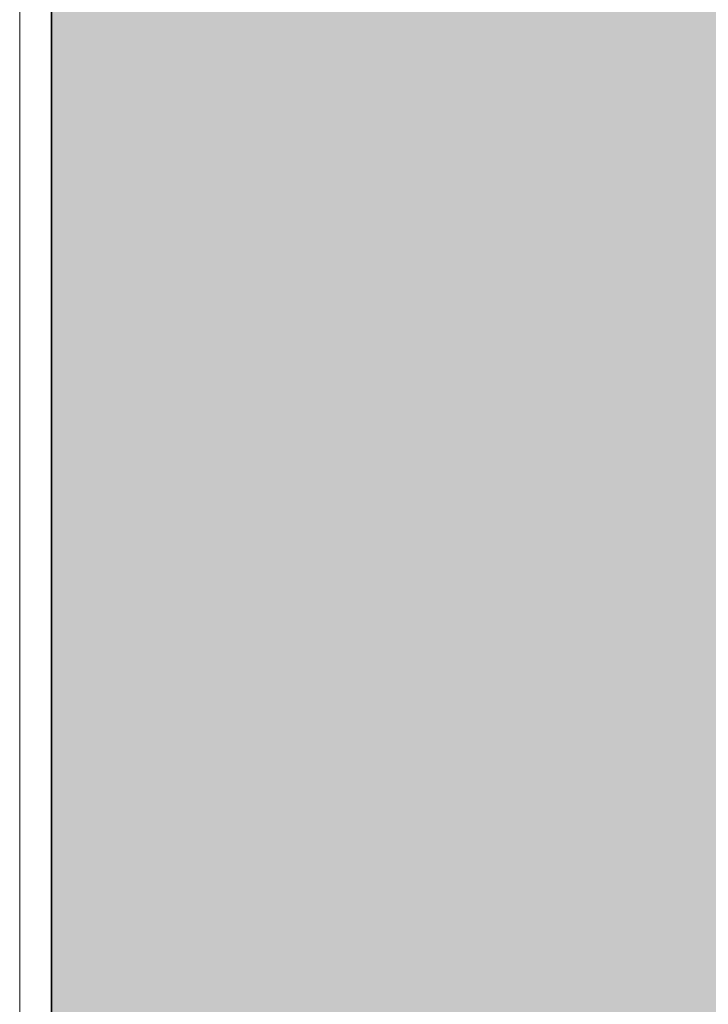
# Model space of a CAD drawing. Units: inches. Extents: x 2091 to 2899, y 967 to 2217.
# Tile 235 of 256: x 2203.1157 to 2203.7172, y 1153.1078 to 1153.9685. Entities that reach past the tile are written whole.
import ezdxf

# ---------------------------------------------------------------- set-up
doc = ezdxf.new("R2010")
doc.units = ezdxf.units.IN
doc.layers.add('A-GLAZ', color=4, linetype='Continuous', lineweight=18)
doc.layers.add('C-PROP', color=7, linetype='Continuous', lineweight=35)
doc.layers.add('A-WALL-PATT', color=141, linetype='Continuous', lineweight=13, true_color=0xadddf7)

# ---------------------------------------------------------------- blocks, each defined once
blk = doc.blocks.new('WIN-DOUBLE-LINE')
blk.add_line((0.0004, -0.00045), (0.0004, 80.8229))

msp = doc.modelspace()

# ---------------------------------------------------------------- hatches: boundary and pattern name
at = {"layer": 'A-WALL-PATT'}
h = msp.add_hatch(color=256, dxfattribs=at)
h.dxf.hatch_style = 1
h.paths.add_polyline_path([(2803.1436, 2050.91906), (2203.1436, 2050.91906), (2203.1436, 1090.91906), (2803.1436, 1090.91906)])
h.paths.add_polyline_path([(2635.79885, 1147.54046), (2674.52405, 1147.54046, 0.376086), (2678.52967, 1152.8802), (2678.52967, 1159.55647, 0.333335), (2674.52432, 1163.56185), (2674.52432, 1163.56185), (2674.52432, 1192.93439), (2635.80597, 1192.93439), (2597.08762, 1192.93439), (2597.08762, 1163.56185, 0.333335), (2593.08228, 1159.55647), (2593.08228, 1152.8802, 0.376086), (2597.08789, 1147.54046)], flags=0)
h.paths.add_polyline_path([(2436.01043, 1278.24078, 0.000483), (2435.95264, 1278.21503, -0.001328), (2435.93563, 1278.11169, -0.001711), (2436.11644, 1278.04076, 0.002185)], flags=0)
h.paths.add_polyline_path([(2794.1436, 1143.41906), (2794.1436, 1347.41906), (2543.37017, 1347.41906), (2543.37017, 1351.91906), (2794.1436, 1351.91906), (2794.1436, 1392.71355), (2793.9474, 1392.71355), (2793.9474, 1473.5369), (2794.1436, 1473.5369), (2794.1436, 1531.91906), (2650.1436, 1531.91906), (2650.1436, 1536.41906), (2794.1436, 1536.41906), (2794.1436, 1692.41906), (2609.37561, 1692.41906), (2609.37561, 1644.41906), (2604.87561, 1644.41906), (2604.87561, 1744.91906), (2609.37561, 1744.91906), (2609.37561, 1696.91906), (2794.1436, 1696.91906), (2794.1436, 1780.91906), (2609.6436, 1780.91906), (2493.87561, 1780.91906), (2493.87561, 1785.41906), (2609.6436, 1785.41906), (2794.1436, 1785.41906), (2794.1436, 1847.93882), (2793.95122, 1847.93882), (2793.95122, 1928.76217), (2794.1436, 1928.76217), (2794.1436, 1941.41906), (2614.1436, 1941.41906), (2614.1436, 1821.41906), (2609.6436, 1821.41906), (2609.6436, 1941.41906), (2392.1436, 1941.41906), (2392.1436, 1819.91906), (2387.6436, 1819.91906), (2387.6436, 1941.41906), (2212.1436, 1941.41906), (2212.1436, 1783.91906), (2392.1436, 1783.91906), (2392.1436, 1780.91906), (2212.1436, 1780.91906), (2212.1436, 1629.41906), (2387.6436, 1629.41906), (2387.6436, 1744.91906), (2392.1436, 1744.91906), (2392.1436, 1627.91906), (2317.1436, 1627.91906), (2317.1436, 1551.41906), (2317.1436, 1536.41906), (2459.38359, 1536.41906), (2459.38359, 1602.39648), (2463.88359, 1602.39648), (2463.88359, 1531.91906), (2456.6436, 1531.91906), (2456.6436, 1529.91906), (2452.1436, 1529.91906), (2452.1436, 1531.91906), (2312.6436, 1531.91906), (2312.6436, 1551.41906), (2306.1436, 1551.41906), (2306.1436, 1555.91906), (2308.1436, 1555.91906), (2308.1436, 1551.41906), (2312.6436, 1551.41906), (2312.6436, 1627.91906), (2212.1436, 1627.91906), (2212.1436, 1555.91906), (2270.1436, 1555.91906), (2270.1436, 1551.41906), (2212.1436, 1551.41906), (2212.1436, 1351.91906), (2272.1436, 1351.91906), (2272.1436, 1347.41906), (2212.1436, 1347.41906), (2212.1436, 1275.41906), (2308.1436, 1275.41906), (2308.1436, 1351.91906), (2452.1436, 1351.91906), (2452.1436, 1493.91906), (2456.6436, 1493.91906), (2456.6436, 1347.41906), (2312.6436, 1347.41906), (2312.6436, 1270.91906), (2212.1436, 1270.91906), (2212.1436, 1099.91906), (2281.23752, 1099.91906), (2282.87104, 1110.9138), (2282.00834, 1116.9966), (2278.55774, 1121.4204), (2268.20564, 1128.0562), (2272.08764, 1128.0562), (2273.81294, 1131.927), (2279.42034, 1134.6919), (2285.02784, 1135.2449), (2287.61584, 1137.4568), (2288.04714, 1138.0098), (2289.34114, 1140.7747), (2291.06654, 1139.6687), (2292.36054, 1135.2449), (2295.37984, 1136.9038), (2296.24254, 1135.7979), (2297.10524, 1133.033), (2300.12464, 1138.0098), (2303.14394, 1138.0098), (2304.43794, 1135.7979), (2303.14394, 1133.586), (2306.59464, 1134.6919), (2307.88874, 1133.033), (2310.90804, 1135.2449), (2313.92744, 1134.1389), (2315.62686, 1132.4271), (2308.32004, 1117.5496), (2290.20384, 1109.8079), (2288.90984, 1103.1721), (2289.27231, 1099.91906), (2434.91823, 1099.91906), (2431.59323, 1124.78806), (2429.93023, 1169.55306), (2430.92718, 1240.51969), (2435.65893, 1238.18613), (2437.13523, 1196.55406), (2438.79823, 1143.97306), (2442.67823, 1111.99806), (2446.55823, 1099.91906), (2794.1436, 1099.91906), (2794.1436, 1138.91906), (2548.03245, 1138.91906), (2548.03245, 1143.41906), (2548.03245, 1148.81906), (2546.66846, 1148.03156), (2528.68569, 1179.17862, 0.256256), (2512.03245, 1148.81906), (2512.03245, 1143.41906), (2512.03245, 1138.91906), (2507.53245, 1138.91906), (2507.53245, 1143.41906), (2507.53245, 1148.81906, 0.256256), (2490.8792, 1179.17862), (2472.89644, 1148.03156), (2471.53245, 1148.81906), (2471.53245, 1143.41906), (2467.03245, 1143.41906), (2467.03245, 1269.94579, 0.039061), (2460.90999, 1273.58006), (2467.03245, 1273.58006), (2467.03245, 1286.32536, 0.014511), (2465.21619, 1286.76191), (2467.03245, 1287.05258), (2467.03245, 1323.41906), (2471.53245, 1323.41906), (2471.53245, 1148.81906), (2489.53245, 1179.99597), (2490.89644, 1179.20847), (2490.8792, 1179.17862, -0.256256), (2507.53245, 1148.81906), (2507.53245, 1143.41906), (2512.03245, 1143.41906), (2512.03245, 1148.81906, -0.256256), (2528.68569, 1179.17862), (2528.66846, 1179.20847), (2530.03245, 1179.99597), (2548.03245, 1148.81906), (2548.03245, 1143.41906)], flags=16)
h.paths.add_polyline_path([(2607.76855, 1200.94508), (2607.76855, 1265.03063), (2597.08762, 1281.05201), (2619.78459, 1281.05201), (2627.79528, 1337.12686), (2635.79885, 1337.12686), (2643.81666, 1337.12686), (2651.82736, 1281.05201), (2674.52432, 1281.05201), (2663.8434, 1265.03063), (2663.8434, 1200.94508), (2635.80597, 1200.94508)], flags=0)
edge = h.paths.add_edge_path(flags=0)
edge.add_ellipse((13303.89622, 1272.99872), major_axis=(-10595.31304, 0), ratio=0.84230387009, start_angle=0.628237219, end_angle=0.6465541, ccw=False)
edge.add_ellipse((2711.70045, 1156.85268), major_axis=(2.21977, 0), ratio=0.8423039, start_angle=111.53524, end_angle=180.62824, ccw=False)
edge.add_ellipse((13303.15629, 1272.99872), major_axis=(-10593.02631, 0), ratio=0.84230386954, start_angle=0.528271472, end_angle=0.646554097, ccw=False)
edge.add_line((2710.7646, 1175.3333), (2710.12999, 1175.3333))
edge.add_ellipse((2710.12999, 1176.57978), major_axis=(1.47985, 0), ratio=0.8423039, start_angle=180, end_angle=270, ccw=False)
edge.add_line((2708.65014, 1176.57978), (2708.65014, 1200.78291))
edge.add_ellipse((2710.12999, 1200.78291), major_axis=(1.47985, 0), ratio=0.8423039, start_angle=90, end_angle=180, ccw=False)
edge.add_line((2710.12999, 1202.02939), (2710.46508, 1202.02939))
edge.add_ellipse((13303.15629, 1272.99872), major_axis=(-10593.02631, 0), ratio=0.84230386954, start_angle=-0.090229089, end_angle=0.383866779, ccw=False)
edge.add_ellipse((2710.12999, 1290.92703), major_axis=(-1.47985, 0), ratio=0.8423039, start_angle=0, end_angle=90, ccw=False)
edge.add_line((2708.65014, 1290.92703), (2708.65014, 1315.13017))
edge.add_ellipse((2710.12999, 1315.13017), major_axis=(-1.47985, 0), ratio=0.8423039, start_angle=-90, end_angle=0, ccw=False)
edge.add_line((2710.12999, 1316.37665), (2710.70631, 1316.37665))
edge.add_ellipse((3238.40172, 1296.28957), major_axis=(528.234, 0), ratio=0.84230387, start_angle=176.3495724, end_angle=177.8200497, ccw=False)
edge.add_ellipse((2775.06304, 1071.4507), major_axis=(313.30776, 0), ratio=0.84230387, start_angle=102.1259656, end_angle=103.780529, ccw=False)
edge.add_ellipse((2775.06304, 1078.3057), major_axis=(-305.30289, 0), ratio=0.84230387, start_angle=-79.790461, end_angle=-77.5553727, ccw=False)
edge.add_ellipse((2695.14177, 1541.97538), major_axis=(-250.96022, 0), ratio=0.84230387, start_angle=99.256566, end_angle=102.5549326)
edge.add_line((2741.41033, 1334.21426), (2747.13255, 1337.37848))
edge.add_ellipse((2747.53862, 1336.85748), major_axis=(-0.73992, 0), ratio=0.842304, start_angle=270, end_angle=307.93313, ccw=False)
edge.add_ellipse((2747.53862, 1336.85748), major_axis=(-0.73992, 0), ratio=0.842304, start_angle=232.06687, end_angle=270, ccw=False)
edge.add_line((2747.94469, 1337.37848), (2753.66691, 1334.21426))
edge.add_ellipse((2799.93547, 1541.97538), major_axis=(250.96022, 0), ratio=0.84230387, start_angle=257.4450674, end_angle=260.743434)
edge.add_ellipse((2720.01419, 1078.3057), major_axis=(305.30289, 0), ratio=0.84230387, start_angle=77.5553727, end_angle=79.790461, ccw=False)
edge.add_ellipse((2720.01419, 1071.4507), major_axis=(-313.30776, 0), ratio=0.84230387, start_angle=256.219471, end_angle=257.8740344, ccw=False)
edge.add_ellipse((2256.67551, 1296.28957), major_axis=(-528.234, 0), ratio=0.84230387, start_angle=182.1799503, end_angle=183.6504276, ccw=False)
edge.add_line((2784.37092, 1316.37665), (2784.94725, 1316.37665))
edge.add_ellipse((2784.94725, 1315.13017), major_axis=(1.47985, 0), ratio=0.8423039, start_angle=0, end_angle=90, ccw=False)
edge.add_line((2786.42709, 1315.13017), (2786.42709, 1290.92703))
edge.add_ellipse((2784.94725, 1290.92703), major_axis=(1.47985, 0), ratio=0.8423039, start_angle=270, end_angle=360, ccw=False)
edge.add_ellipse((-7808.07906, 1272.99872), major_axis=(10593.02631, 0), ratio=0.84230386954, start_angle=-0.383866779, end_angle=0.090229089, ccw=False)
edge.add_line((2784.61216, 1202.02939), (2784.94725, 1202.02939))
edge.add_ellipse((2784.94725, 1200.78291), major_axis=(1.47985, 0), ratio=0.8423039, start_angle=0, end_angle=90, ccw=False)
edge.add_line((2786.42709, 1200.78291), (2786.42709, 1176.57978))
edge.add_ellipse((2784.94725, 1176.57978), major_axis=(-1.47985, 0), ratio=0.8423039, start_angle=90, end_angle=180, ccw=False)
edge.add_line((2784.94725, 1175.3333), (2784.31264, 1175.3333))
edge.add_ellipse((-7808.07906, 1272.99872), major_axis=(10593.02631, 0), ratio=0.84230386954, start_angle=-0.618643196, end_angle=-0.528271472, ccw=False)
edge.add_ellipse((2783.37678, 1156.85268), major_axis=(-2.21977, 0), ratio=0.8423039, start_angle=179.37176, end_angle=248.46476, ccw=False)
edge.add_ellipse((-7808.81898, 1272.99872), major_axis=(-10595.31304, 0), ratio=0.84230386576, start_angle=179.353445923, end_angle=179.371762803, ccw=False)
edge.add_ellipse((2780.2973, 1153.50079), major_axis=(-5.24643, 0), ratio=0.8423039, start_angle=90, end_angle=179.35345, ccw=False)
edge.add_line((2780.2973, 1149.08171), (2714.77993, 1149.08171))
edge.add_ellipse((2714.77993, 1153.50079), major_axis=(5.24643, 0), ratio=0.8423039, start_angle=180.64655, end_angle=270, ccw=False)
edge = h.paths.add_edge_path(flags=0)
edge.add_line((2718.18737, 1151.00783), (2718.18737, 1170.47236))
edge.add_ellipse((2721.14706, 1170.47236), major_axis=(-2.95969, 0), ratio=0.8423039, start_angle=-90, end_angle=0, ccw=False)
edge.add_line((2721.14706, 1172.96532), (2773.93017, 1172.96532))
edge.add_ellipse((2773.93017, 1170.47236), major_axis=(-2.95969, 0), ratio=0.8423039, start_angle=180, end_angle=270, ccw=False)
edge.add_line((2776.88987, 1170.47236), (2776.88987, 1151.00783))
edge.add_line((2776.88987, 1151.00783), (2718.18737, 1151.00783))
edge = h.paths.add_edge_path(flags=0)
edge.add_line((2718.18737, 1180.23415), (2718.18737, 1199.05783))
edge.add_ellipse((2747.53862, 1320.39864), major_axis=(147.01792, 0), ratio=0.84230387, start_angle=256.4018653, end_angle=283.5981347)
edge.add_line((2776.88987, 1199.05783), (2776.88987, 1180.23415))
edge.add_ellipse((2747.53862, 1301.57496), major_axis=(147.01792, 0), ratio=0.84230387, start_angle=256.4018653, end_angle=283.5981347, ccw=False)
edge = h.paths.add_edge_path(flags=0)
edge.add_ellipse((13303.15629, 1272.99872), major_axis=(-10591.54646, 0), ratio=0.84230386955, start_angle=0.055594314, end_angle=0.377764194, ccw=False)
edge.add_line((2711.61686, 1262.72171), (2715.66741, 1249.4954))
edge.add_ellipse((6413.89196, 1241.69192), major_axis=(-3698.23616, 0), ratio=0.8423038695, start_angle=-0.12089737, end_angle=0.36407635)
edge.add_line((2715.76104, 1218.19245), (2711.93431, 1203.16736))
edge = h.paths.add_edge_path(flags=0)
edge.add_line((2718.18737, 1251.07457), (2716.00249, 1267.45044))
edge.add_ellipse((2742.15117, 1202.18954), major_axis=(81.77258, 0), ratio=0.84230387, start_angle=94.277421, end_angle=111.8349538, ccw=False)
edge.add_line((2737.00975, 1270.93063), (2758.06748, 1270.93063))
edge.add_ellipse((2752.92606, 1202.18954), major_axis=(81.77258, 0), ratio=0.84230387, start_angle=68.1650462, end_angle=85.722579, ccw=False)
edge.add_line((2779.07475, 1267.45044), (2776.88987, 1251.07457))
edge.add_ellipse((2750.33806, 1187.88536), major_axis=(79.57966, 0), ratio=0.84230387, start_angle=67.2080851, end_angle=85.1299304)
edge.add_line((2756.03466, 1254.74366), (2739.04258, 1254.74366))
edge.add_ellipse((2744.73917, 1187.88536), major_axis=(79.57966, 0), ratio=0.84230387, start_angle=94.8700696, end_angle=112.7919149)
edge = h.paths.add_edge_path(flags=0)
edge.add_line((2783.14293, 1203.16736), (2779.31619, 1218.19245))
edge.add_ellipse((-918.81473, 1241.69192), major_axis=(3698.23616, 0), ratio=0.8423038695, start_angle=-0.36407635, end_angle=0.12089737)
edge.add_line((2779.40983, 1249.4954), (2783.46037, 1262.72171))
edge.add_ellipse((-7808.07906, 1272.99872), major_axis=(-10591.54646, 0), ratio=0.84230386954, start_angle=179.622235806, end_angle=179.944405687, ccw=False)
edge = h.paths.add_edge_path(flags=0)
edge.add_ellipse((2734.20089, 1286.69044), major_axis=(-0.35661, 6.34008), ratio=0.6038336, start_angle=89.002014, end_angle=253.657408, ccw=False)
edge.add_line((2730.369, 1286.54181), (2730.369, 1301.35198))
edge.add_line((2730.369, 1301.35198), (2735.91331, 1305.2148))
edge.add_ellipse((2736.38492, 1304.73456), major_axis=(0.73992, 0), ratio=0.842304, start_angle=90, end_angle=134.48021, ccw=False)
edge.add_line((2736.38492, 1305.3578), (2738.03278, 1305.3578))
edge.add_line((2738.03278, 1305.3578), (2738.03278, 1307.70793))
edge.add_ellipse((2794.20164, 1307.70793), major_axis=(56.16886, 0), ratio=0.84230387, start_angle=150.56143, end_angle=180, ccw=False)
edge.add_ellipse((2700.87559, 1307.70793), major_axis=(-56.16886, 0), ratio=0.84230387, start_angle=180, end_angle=209.43857, ccw=False)
edge.add_line((2757.04445, 1307.70793), (2757.04445, 1305.3578))
edge.add_line((2757.04445, 1305.3578), (2758.69232, 1305.3578))
edge.add_ellipse((2758.69232, 1304.73456), major_axis=(-0.73992, 0), ratio=0.842304, start_angle=225.51979, end_angle=270, ccw=False)
edge.add_line((2759.16392, 1305.2148), (2764.70823, 1301.35198))
edge.add_line((2764.70823, 1301.35198), (2764.70823, 1286.54181))
edge.add_ellipse((2760.87634, 1286.69044), major_axis=(0.35661, 6.34008), ratio=0.6038336, start_angle=106.342592, end_angle=270.997986, ccw=False)
edge.add_line((2757.04445, 1285.79709), (2757.04445, 1307.70793))
edge.add_ellipse((2700.87559, 1307.70793), major_axis=(-56.16886, 0), ratio=0.84230387, start_angle=180, end_angle=209.43857)
edge.add_ellipse((2794.20164, 1307.70793), major_axis=(56.16886, 0), ratio=0.84230387, start_angle=150.56143, end_angle=180)
edge.add_line((2738.03278, 1307.70793), (2738.03278, 1285.79709))
h.paths.add_polyline_path([(2417.81227, 1104.4497), (2413.49227, 1102.5297), (2410.61227, 1103.9697), (2409.17227, 1106.3697), (2407.25227, 1107.3297), (2406.29227, 1109.7297), (2405.33227, 1114.0497), (2405.33227, 1117.8897), (2406.29227, 1120.1297), (2407.25227, 1119.8097), (2408.84832, 1118.32766), (2410.17395, 1119.42417), (2410.21127, 1120.4057), (2411.04073, 1121.41905), (2410.69927, 1119.8587), (2410.17395, 1119.42417), (2410.08845, 1117.17611), (2411.13284, 1116.20632), (2413.97227, 1119.3297), (2416.85227, 1120.7697), (2416.86972, 1120.79878), (2417.03507, 1119.40512), (2417.89621, 1118.14338), (2418.29227, 1118.3697), (2419.54445, 1120.03927), (2419.36092, 1118.38749), (2419.03211, 1119.35615), (2418.39894, 1118.51193), (2419.25227, 1114.5297), (2418.79409, 1107.19879)], flags=0)
h.paths.add_polyline_path([(2508.87017, 1347.41906), (2508.37017, 1347.41906), (2508.37017, 1351.91906), (2508.87017, 1351.91906)], flags=0)
h.paths.add_polyline_path([(2473.37017, 1347.41906), (2472.37017, 1347.41906), (2467.87017, 1347.41906), (2467.87017, 1455.41906), (2472.37017, 1455.41906), (2472.37017, 1352.41906), (2473.37017, 1352.41906)], flags=0)
h.paths.add_polyline_path([(2352.10624, 1217.4462), (2349.22624, 1218.8862), (2347.78624, 1221.2862), (2345.86624, 1222.2462), (2344.90624, 1224.6462), (2343.94624, 1228.9662), (2343.94624, 1232.8062), (2344.90624, 1235.0462), (2345.86624, 1234.7262), (2347.46229, 1233.24415), (2348.78792, 1234.34066), (2348.82524, 1235.3222), (2349.6547, 1236.33555), (2349.31324, 1234.7752), (2348.78792, 1234.34066), (2348.70242, 1232.0926), (2349.74681, 1231.12282), (2352.58624, 1234.2462), (2355.46624, 1235.6862), (2355.48369, 1235.71528), (2355.64904, 1234.32161), (2356.51018, 1233.05988), (2356.90624, 1233.2862), (2358.15842, 1234.95576), (2357.97489, 1233.30398), (2357.64608, 1234.27264), (2357.01291, 1233.42842), (2357.86624, 1229.4462), (2357.40806, 1222.11529), (2356.42624, 1219.3662)], flags=0)
h.paths.add_polyline_path([(2348.2968, 1112.22442), (2347.0138, 1112.31042), (2345.5298, 1114.12742), (2345.7318, 1115.85842), (2346.8118, 1116.98242), (2346.8118, 1114.64642), (2345.8668, 1114.21442), (2346.8798, 1114.30042)], flags=0)
h.paths.add_polyline_path([(2347.0138, 1110.92642), (2346.2718, 1110.49342), (2346.6098, 1111.18642)], flags=0)
h.paths.add_polyline_path([(2345.8668, 1118.19442), (2345.5298, 1117.32942), (2343.7078, 1118.02142), (2344.3828, 1118.62642)], flags=0)
h.paths.add_polyline_path([(2346.6768, 1109.28242), (2346.0698, 1108.07142), (2345.8668, 1110.06142)], flags=0)
h.paths.add_polyline_path([(2345.0568, 1119.75142), (2343.6398, 1119.75142), (2343.9778, 1121.13542)], flags=0)
h.paths.add_polyline_path([(2345.2598, 1116.55042), (2345.1248, 1115.85842), (2344.9218, 1115.68542), (2344.7198, 1116.37742)], flags=0)
h.paths.add_polyline_path([(2345.6648, 1112.31042), (2345.4618, 1111.53242), (2344.0448, 1111.96442), (2344.6518, 1112.57042)], flags=0)
h.paths.add_polyline_path([(2345.1918, 1113.34942), (2344.4498, 1113.86842), (2344.7198, 1114.38742)], flags=0)
h.paths.add_polyline_path([(2344.6518, 1116.80942), (2344.1798, 1115.68542), (2344.6518, 1115.33942), (2343.9098, 1114.90642), (2343.0328, 1115.94442), (2343.6398, 1116.46342)], flags=0)
h.paths.add_polyline_path([(2345.8668, 1106.68642), (2344.9898, 1105.56242), (2344.5168, 1106.60042)], flags=0)
h.paths.add_polyline_path([(2344.8548, 1110.06142), (2344.5168, 1109.28242), (2344.1128, 1109.71542)], flags=0)
h.paths.add_polyline_path([(2344.0448, 1113.52242), (2343.4378, 1113.08942), (2342.7628, 1113.95442)], flags=0)
h.paths.add_polyline_path([(2344.3148, 1111.01242), (2342.9648, 1110.32042), (2342.9648, 1111.09942)], flags=0)
h.paths.add_polyline_path([(2345.1248, 1104.69742), (2344.5848, 1103.74542), (2344.4498, 1104.26442)], flags=0)
h.paths.add_polyline_path([(2342.8298, 1121.22242), (2341.7498, 1120.53042), (2340.5358, 1121.04942), (2340.1308, 1121.82842), (2340.6708, 1122.95242), (2341.1428, 1121.82842), (2341.6148, 1122.00142)], flags=0)
h.paths.add_polyline_path([(2342.9648, 1119.75142), (2343.0328, 1118.45342), (2342.0878, 1118.02142), (2342.0198, 1119.49142)], flags=0)
h.paths.add_polyline_path([(2342.6948, 1116.89642), (2341.9528, 1116.63642), (2342.0198, 1117.32942)], flags=0)
h.paths.add_polyline_path([(2343.0328, 1112.22442), (2342.0198, 1111.79142), (2341.5478, 1112.22442), (2342.3578, 1113.34942)], flags=0)
h.paths.add_polyline_path([(2343.7748, 1104.43742), (2342.6278, 1102.88042), (2342.6948, 1104.61042), (2343.4378, 1105.12942)], flags=0)
h.paths.add_polyline_path([(2342.0198, 1115.07942), (2340.8058, 1115.51242), (2340.9408, 1116.37742)], flags=0)
h.paths.add_polyline_path([(2341.4808, 1120.09742), (2341.4808, 1119.40542), (2341.0758, 1119.57842), (2341.1428, 1120.09742)], flags=0)
h.paths.add_polyline_path([(2341.8178, 1114.47342), (2340.9408, 1113.08942), (2340.8058, 1114.56042)], flags=0)
h.paths.add_polyline_path([(2341.1428, 1118.54042), (2340.9408, 1116.98242), (2339.0508, 1117.67542), (2339.0508, 1118.62642)], flags=0)
h.paths.add_polyline_path([(2342.6948, 1101.66842), (2341.9528, 1101.84142), (2342.5598, 1102.36142)], flags=0)
h.paths.add_polyline_path([(2340.3328, 1119.66542), (2338.4438, 1119.57842), (2337.9038, 1120.35742), (2339.6578, 1120.61642)], flags=0)
h.paths.add_polyline_path([(2340.3328, 1115.33942), (2340.0628, 1113.69542), (2339.3878, 1115.33942)], flags=0)
h.paths.add_polyline_path([(2341.8178, 1103.83142), (2341.5478, 1102.88042), (2341.1428, 1103.65842)], flags=0)
h.paths.add_polyline_path([(2339.0508, 1122.86642), (2337.2958, 1121.82842), (2337.0938, 1123.12542), (2337.7688, 1123.81842)], flags=0)
h.paths.add_polyline_path([(2339.1178, 1121.74142), (2338.8478, 1121.22242), (2338.1738, 1121.04942), (2338.3758, 1121.56842)], flags=0)
h.paths.add_polyline_path([(2339.1858, 1119.31942), (2338.6458, 1118.71342), (2338.2408, 1118.10742), (2338.2408, 1118.88642)], flags=0)
h.paths.add_polyline_path([(2341.1428, 1101.92842), (2340.6028, 1101.23642), (2340.0628, 1101.84142), (2340.6028, 1102.36142)], flags=0)
h.paths.add_polyline_path([(2337.6338, 1117.76142), (2336.6208, 1118.28042), (2337.2958, 1118.97242)], flags=0)
h.paths.add_polyline_path([(2336.8238, 1119.57842), (2334.7988, 1118.97242), (2335.2038, 1120.35742), (2336.5538, 1120.87642)], flags=0)
h.paths.add_polyline_path([(2339.1178, 1100.45742), (2337.3638, 1100.54342), (2336.7558, 1101.23642)], flags=0)
h.paths.add_polyline_path([(2336.3508, 1122.43342), (2336.0138, 1121.91442), (2334.9338, 1122.43342), (2334.5288, 1123.47142), (2335.7438, 1122.77942)], flags=0)
h.paths.add_polyline_path([(2334.7318, 1120.87642), (2334.2588, 1120.35742), (2334.0568, 1120.78942), (2334.5968, 1121.30842)], flags=0)
h.paths.add_polyline_path([(2334.4618, 1122.17442), (2332.5718, 1121.30842), (2331.3568, 1122.17442), (2332.0998, 1122.86642)], flags=0)
h.paths.add_polyline_path([(2334.2588, 1118.54042), (2333.3818, 1118.45342), (2333.6518, 1119.31942)], flags=0)
h.paths.add_polyline_path([(2335.5418, 1102.27442), (2334.1918, 1102.62042), (2335.2718, 1103.31242)], flags=0)
h.paths.add_polyline_path([(2332.7068, 1119.66542), (2331.6948, 1120.44342), (2332.5048, 1120.78942)], flags=0)
h.paths.add_polyline_path([(2334.7318, 1101.14942), (2333.5168, 1101.58242), (2333.9888, 1101.75542)], flags=0)
h.paths.add_polyline_path([(2332.6398, 1116.63642), (2331.0868, 1116.29042), (2331.9648, 1118.19442)], flags=0)
h.paths.add_polyline_path([(2330.7498, 1121.56842), (2330.2768, 1120.27042), (2328.5228, 1119.31942), (2328.9948, 1121.04942)], flags=0)
h.paths.add_polyline_path([(2330.7498, 1118.62642), (2330.0078, 1117.50242), (2329.8728, 1118.02142)], flags=0)
h.paths.add_polyline_path([(2332.0998, 1102.36142), (2330.5468, 1102.01442), (2331.6948, 1102.96642)], flags=0)
h.paths.add_polyline_path([(2329.5348, 1113.60842), (2329.0628, 1112.31042), (2328.5898, 1113.34942)], flags=0)
h.paths.add_polyline_path([(2328.3878, 1117.84842), (2327.5098, 1116.55042), (2327.1728, 1117.76142)], flags=0)
h.paths.add_polyline_path([(2329.7378, 1106.51342), (2329.5348, 1105.30242), (2328.2528, 1106.08142)], flags=0)
h.paths.add_polyline_path([(2328.6578, 1114.38742), (2328.0498, 1114.12742), (2328.3198, 1114.90642)], flags=0)
h.paths.add_polyline_path([(2328.3198, 1112.22442), (2327.1058, 1112.13742), (2326.7008, 1112.65642)], flags=0)
h.paths.add_polyline_path([(2326.9028, 1115.25242), (2326.7008, 1114.12742), (2325.2158, 1113.60842), (2326.0928, 1115.33942)], flags=0)
h.paths.add_polyline_path([(2326.6328, 1108.33042), (2326.0928, 1107.37942), (2325.8908, 1108.50342), (2326.4978, 1109.10942)], flags=0)
h.paths.add_polyline_path([(2615.1436, 1531.91906), (2609.6436, 1531.91906), (2609.6436, 1620.41906), (2614.1436, 1620.41906), (2614.1436, 1536.41906), (2615.1436, 1536.41906)], flags=0)
h.paths.add_polyline_path([(2545.1436, 1563.41906), (2464.1436, 1563.41906), (2464.1436, 1632.41906), (2509.1436, 1632.41906), (2509.1436, 1627.91906), (2509.1436, 1603.91906), (2468.6436, 1603.91906), (2468.6436, 1567.91906), (2540.6436, 1567.91906), (2540.6436, 1591.91906), (2545.1436, 1591.91906)], flags=0)
h.paths.add_polyline_path([(2388.96905, 1549.98573), (2357.43418, 1549.98573), (2357.43418, 1623.36078), (2399.36278, 1623.36078), (2435.68947, 1623.36078), (2435.59255, 1602.55927), (2435.59255, 1602.39648), (2388.96905, 1602.39648)], flags=0)
h.paths.add_polyline_path([(2388.88063, 1555.80915), (2374.90443, 1555.80915), (2374.90443, 1600.57156), (2374.90443, 1615.45765), (2406.35088, 1615.45765), (2406.35088, 1618.93943), (2412.17429, 1615.45765), (2406.35088, 1611.97586), (2406.35088, 1615.45765), (2388.88063, 1615.45765)], flags=0)
h.paths.add_polyline_path([(2568.87561, 1644.41906), (2453.37561, 1644.41906), (2453.37561, 1785.41906), (2457.87561, 1785.41906), (2457.87561, 1648.91906), (2568.87561, 1648.91906)], flags=0)
h.paths.add_polyline_path([(2212.1436, 1945.91906), (2212.1436, 2041.91906), (2794.1436, 2041.91906), (2794.1436, 1945.91906)], flags=16)
h.paths.add_polyline_path([(2271.08273, 1964.31724), (2776.85297, 1964.31724), (2776.85297, 2037.16962), (2271.08273, 2037.16962)], flags=8)
h.paths.add_polyline_path([(2380.64929, 1536.82414), (2461.04081, 1536.82414), (2461.04081, 1554.65259), (2380.64929, 1554.65259)], flags=8)
h.paths.add_polyline_path([(2240.75571, 1609.72545), (2309.18583, 1609.72545), (2309.18583, 1617.6982), (2240.75571, 1617.6982)], flags=8)
h.paths.add_polyline_path([(2212.67726, 1313.5041), (2282.59152, 1313.5041), (2282.59152, 1322.74524), (2212.67726, 1322.74524)], flags=8)
h.paths.add_polyline_path([(2457.11198, 1114.77857), (2558.48158, 1114.77857), (2558.48158, 1142.21968), (2457.11198, 1142.21968)], flags=8)
h.paths.add_polyline_path([(2473.44234, 1273.01007), (2604.64123, 1273.01007), (2604.64123, 1318.34693), (2473.44234, 1318.34693)], flags=8)
h.paths.add_polyline_path([(2638.8763, 1626.97743), (2684.25037, 1627.97674), (2684.03848, 1637.59749), (2638.66442, 1636.59819)], flags=8)
h.paths.add_polyline_path([(2537.59055, 1453.79345), (2628.38955, 1453.79345), (2628.38955, 1475.34481), (2537.59055, 1475.34481)], flags=8)
h.paths.add_polyline_path([(2504.13764, 1714.6324), (2554.64719, 1714.6324), (2554.64719, 1730.23771), (2504.13764, 1730.23771)], flags=8)
h.paths.add_polyline_path([(2487.50118, 1575.65187), (2535.09712, 1575.65187), (2535.09712, 1598.37765), (2487.50118, 1598.37765)], flags=8)
h.paths.add_polyline_path([(2709.0994, 1735.71028), (2740.0166, 1735.71028), (2740.0166, 1749.93764), (2709.0994, 1749.93764)], flags=8)
h.paths.add_polyline_path([(2442.43842, 1792.17166), (2564.72884, 1792.17166), (2564.72884, 1842.00016), (2442.43842, 1842.00016)], flags=8)
h.paths.add_polyline_path([(2655.8158, 1809.64408), (2789.52014, 1806.6938), (2790.08498, 1832.29164), (2656.38064, 1835.24192)], flags=8)
h.paths.add_polyline_path([(2234.8427, 1797.72014), (2368.59285, 1794.76885), (2369.16072, 1820.50413), (2235.41056, 1823.45542)], flags=8)
h.paths.add_polyline_path([(2245.13847, 1644.00633), (2398.42773, 1640.6239), (2398.99484, 1666.32482), (2245.70557, 1669.70725)], flags=8)
h.paths.add_polyline_path([(2306.14285, 1431.16852), (2413.76831, 1428.79369), (2414.33315, 1454.39153), (2306.70768, 1456.76636)], flags=8)
h.paths.add_polyline_path([(2306.83458, 1458.23314), (2393.38048, 1456.32345), (2393.93281, 1481.35436), (2307.38691, 1483.26405)], flags=8)

# ---------------------------------------------------------------- linework, layer by layer
at = {"layer": 'C-PROP'}
msp.add_lwpolyline([(2203.1436, 2050.91906), (2803.1436, 2050.91906), (2803.1436, 1090.91906), (2203.1436, 1090.91906)], close=True, dxfattribs=at)

# ---------------------------------------------------------------- block references
at = {"layer": 'A-GLAZ'}
msp.add_blockref('WIN-DOUBLE-LINE', (2203.11534, 1152.2475), dxfattribs=at)

doc.saveas('drawing.dxf')
